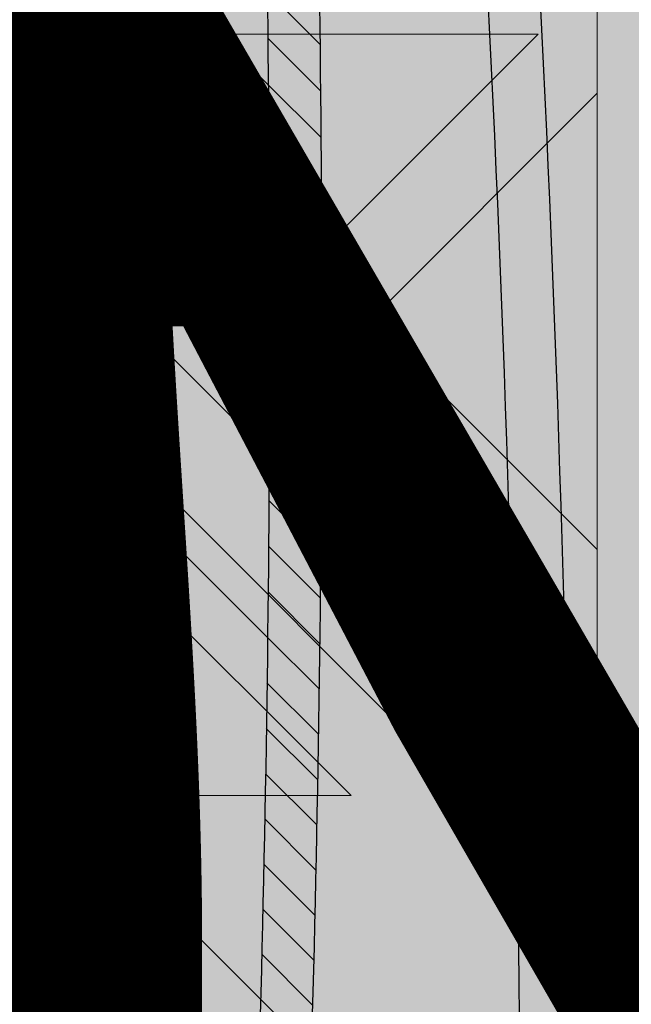
# Model space of a CAD drawing. Units: inches. Extents: x 844 to 2234, y 346 to 1084.
# Tile 82 of 93: x 2006.557 to 2008.425, y 701.365 to 704.373. Entities that reach past the tile are written whole.
import ezdxf

# ---------------------------------------------------------------- set-up
doc = ezdxf.new("R2010")
doc.units = ezdxf.units.IN
doc.header["$MEASUREMENT"] = 0
for name, color, linetype, lineweight in [('A-ANNO-DIMS', 2, 'Continuous', 18), ('furniture', 8, 'Continuous', 18), ('RA-AP-01$0$INT', 35, 'Continuous', 5)]:
    doc.layers.add(name, color=color, linetype=linetype, lineweight=lineweight)
doc.layers.add('RA-AP-01$0$FURN', color=3, linetype='Continuous')
doc.layers.add('RA-AP-01$0$WOOD', color=64, linetype='Continuous')
doc.styles.get("Standard").update_dxf_attribs({"font": 'arial.ttf'})
doc.dimstyles.get("Standard").update_dxf_attribs({"dimtxt": 6, "dimasz": 3, "dimexe": 0.18, "dimexo": 0.0625, "dimgap": 0.09, "dimtad": 0, "dimtih": 1, "dimtoh": 1, "dimdec": 1, "dimzin": 0, "dimdsep": 46, "dimlunit": 3, "dimtxsty": 'Standard', "dimblk": 'ARCHTICK', "dimcen": 0.09, "dimadec": 0, "dimazin": 0, "dimtfac": 1, "dimtdec": 1, "dimtofl": 0, "dimtmove": 0, "dimatfit": 3, "dimfxl": 1, "dimtolj": 1, "dimtzin": 0, "dimarcsym": 0})

# ---------------------------------------------------------------- blocks, each defined once
blk = doc.blocks.new('A$C18D01794')
at = {"layer": 'RA-AP-01$0$INT'}
for points in [[(4.50521, -6.30671), (5.30521, -6.30671), (5.30521, -7.10671), (5.25521, -7.10671), (5.25521, -6.35671), (4.55521, -6.35671), (4.55521, -7.10671), (4.50521, -7.10671)], [(4.50521, -7.90671), (5.30521, -7.90671), (5.30521, -7.10671), (5.25521, -7.10671), (5.25521, -7.85671), (4.55521, -7.85671), (4.55521, -7.10671), (4.50521, -7.10671)]]:
    blk.add_hatch(color=256, dxfattribs=at).paths.add_polyline_path(points)
h = blk.add_hatch(color=256, dxfattribs=at)
h.paths.add_polyline_path([(4.58592, -6.35671), (4.6142, -6.35671), (4.66885, -6.41136), (4.72349, -6.35671), (4.77177, -6.35671), (4.82642, -6.41136), (4.86278, -6.375), (4.8445, -6.35671), (4.86278, -6.35671), (4.90521, -6.39914), (4.94763, -6.35671), (4.96592, -6.35671), (4.94763, -6.375), (4.98399, -6.41136), (5.03864, -6.35671), (5.08692, -6.35671), (5.14157, -6.41136), (5.19621, -6.35671), (5.2245, -6.35671), (4.90521, -6.676)])
h.paths.add_polyline_path([(4.89521, -6.63772), (4.89521, -6.52843), (4.84056, -6.58307)], flags=16)
h.paths.add_polyline_path([(4.91521, -6.63772), (4.96985, -6.58307), (4.91521, -6.52843)], flags=16)
h.paths.add_polyline_path([(4.82642, -6.56893), (4.88106, -6.51429), (4.77177, -6.51429)], flags=16)
h.paths.add_polyline_path([(4.98399, -6.56893), (5.03864, -6.51429), (4.92935, -6.51429)], flags=16)
h.paths.add_polyline_path([(4.88106, -6.49429), (4.82642, -6.43964), (4.77177, -6.49429)], flags=16)
h.paths.add_polyline_path([(4.92935, -6.49429), (5.03864, -6.49429), (4.98399, -6.43964)], flags=16)
h.paths.add_polyline_path([(4.89521, -6.48014), (4.89521, -6.40742), (4.87692, -6.38914), (4.84056, -6.4255)], flags=16)
h.paths.add_polyline_path([(4.91521, -6.48014), (4.96985, -6.4255), (4.93349, -6.38914), (4.91521, -6.40742)], flags=16)
h.paths.add_polyline_path([(4.75763, -6.48014), (4.81228, -6.4255), (4.75763, -6.37085)], flags=16)
h.paths.add_polyline_path([(4.73763, -6.48014), (4.73763, -6.37085), (4.68299, -6.4255)], flags=16)
h.paths.add_polyline_path([(5.05278, -6.48014), (5.05278, -6.37085), (4.99814, -6.4255)], flags=16)
h.paths.add_polyline_path([(5.07278, -6.48014), (5.12742, -6.4255), (5.07278, -6.37085)], flags=16)
h.paths.add_polyline_path([(4.93592, -6.70671), (5.25521, -6.38742), (5.25521, -6.41571), (5.20056, -6.47035), (5.25521, -6.525), (5.25521, -6.57328), (5.20056, -6.62793), (5.23692, -6.66429), (5.25521, -6.646), (5.25521, -6.66429), (5.21278, -6.70671), (5.25521, -6.74914), (5.25521, -6.76742), (5.23692, -6.74914), (5.20056, -6.7855), (5.25521, -6.84014), (5.25521, -6.88843), (5.20056, -6.94307), (5.25521, -6.99772), (5.25521, -7.026)])
h.paths.add_polyline_path([(5.04299, -6.7855), (5.09763, -6.84014), (5.09763, -6.73085)], flags=16)
h.paths.add_polyline_path([(5.02885, -6.77136), (5.08349, -6.71671), (4.9742, -6.71671)], flags=16)
h.paths.add_polyline_path([(5.11763, -6.84014), (5.17228, -6.7855), (5.11763, -6.73085)], flags=16)
h.paths.add_polyline_path([(5.08349, -6.69671), (5.02885, -6.64207), (4.9742, -6.69671)], flags=16)
h.paths.add_polyline_path([(5.13177, -6.85429), (5.18642, -6.79964), (5.24106, -6.85429)], flags=17)
h.paths.add_polyline_path([(5.13177, -6.71671), (5.18642, -6.77136), (5.22278, -6.735), (5.2045, -6.71671)], flags=16)
h.paths.add_polyline_path([(5.09763, -6.68257), (5.09763, -6.57328), (5.04299, -6.62793)], flags=16)
h.paths.add_polyline_path([(5.13177, -6.87429), (5.24106, -6.87429), (5.18642, -6.92893)], flags=17)
h.paths.add_polyline_path([(5.13177, -6.69671), (5.2045, -6.69671), (5.22278, -6.67843), (5.18642, -6.64207)], flags=16)
h.paths.add_polyline_path([(5.11763, -6.68257), (5.17228, -6.62793), (5.11763, -6.57328)], flags=16)
h.paths.add_polyline_path([(5.18642, -6.61378), (5.24106, -6.55914), (5.13177, -6.55914)], flags=16)
h.paths.add_polyline_path([(5.13177, -6.53914), (5.24106, -6.53914), (5.18642, -6.48449)], flags=16)
h.paths.add_polyline_path([(5.25521, -7.08742), (5.25521, -7.10671), (4.55521, -7.10671), (4.55521, -7.08742), (4.90521, -6.73742)])
h.paths.add_polyline_path([(4.98399, -6.84449), (4.92935, -6.89914), (5.03864, -6.89914)], flags=16)
h.paths.add_polyline_path([(4.96985, -6.83035), (4.91521, -6.77571), (4.91521, -6.885)], flags=16)
h.paths.add_polyline_path([(4.92935, -6.91914), (4.98399, -6.97378), (5.03864, -6.91914)], flags=16)
h.paths.add_polyline_path([(5.05278, -6.93328), (4.99814, -6.98793), (5.05278, -7.04257)], flags=16)
h.paths.add_polyline_path([(5.07278, -6.93328), (5.07278, -7.04257), (5.12742, -6.98793)], flags=16)
h.paths.add_polyline_path([(4.89521, -6.77571), (4.84056, -6.83035), (4.89521, -6.885)], flags=16)
h.paths.add_polyline_path([(4.91521, -6.93328), (4.91521, -7.006), (4.93349, -7.02429), (4.96985, -6.98793)], flags=16)
h.paths.add_polyline_path([(4.88106, -6.89914), (4.82642, -6.84449), (4.77177, -6.89914)], flags=16)
h.paths.add_polyline_path([(4.89521, -6.93328), (4.84056, -6.98793), (4.87692, -7.02429), (4.89521, -7.006)], flags=16)
h.paths.add_polyline_path([(4.98399, -7.00207), (4.94763, -7.03843), (4.96592, -7.05671), (5.03864, -7.05671)], flags=16)
h.paths.add_polyline_path([(4.88106, -6.91914), (4.77177, -6.91914), (4.82642, -6.97378)], flags=16)
h.paths.add_polyline_path([(4.90521, -7.01429), (4.86278, -7.05671), (4.94763, -7.05671)], flags=16)
h.paths.add_polyline_path([(5.14157, -7.00207), (5.08692, -7.05671), (5.19621, -7.05671)], flags=16)
h.paths.add_polyline_path([(4.82642, -7.00207), (4.77177, -7.05671), (4.8445, -7.05671), (4.86278, -7.03843)], flags=16)
h.paths.add_polyline_path([(4.81228, -6.98793), (4.75763, -6.93328), (4.75763, -7.04257)], flags=16)
h.paths.add_polyline_path([(4.73763, -6.93328), (4.68299, -6.98793), (4.73763, -7.04257)], flags=16)
h.paths.add_polyline_path([(4.72349, -7.05671), (4.66885, -7.00207), (4.6142, -7.05671)], flags=16)
h.paths.add_polyline_path([(4.59763, -6.70671), (4.55521, -6.66429), (4.55521, -6.646), (4.57349, -6.66429), (4.60985, -6.62793), (4.55521, -6.57328), (4.55521, -6.525), (4.60985, -6.47035), (4.55521, -6.41571), (4.55521, -6.38742), (4.8745, -6.70671), (4.55521, -7.026), (4.55521, -6.99772), (4.60985, -6.94307), (4.55521, -6.88843), (4.55521, -6.84014), (4.60985, -6.7855), (4.57349, -6.74914), (4.55521, -6.76742), (4.55521, -6.74914)])
h.paths.add_polyline_path([(4.71278, -6.73085), (4.71278, -6.84014), (4.76742, -6.7855)], flags=16)
h.paths.add_polyline_path([(4.72692, -6.71671), (4.78157, -6.77136), (4.83621, -6.71671)], flags=16)
h.paths.add_polyline_path([(4.69278, -6.73085), (4.63814, -6.7855), (4.69278, -6.84014)], flags=16)
h.paths.add_polyline_path([(4.72692, -6.69671), (4.83621, -6.69671), (4.78157, -6.64207)], flags=16)
h.paths.add_polyline_path([(4.67864, -6.71671), (4.60592, -6.71671), (4.58763, -6.735), (4.62399, -6.77136)], flags=16)
h.paths.add_polyline_path([(4.71278, -6.68257), (4.76742, -6.62793), (4.71278, -6.57328)], flags=16)
h.paths.add_polyline_path([(4.67864, -6.69671), (4.62399, -6.64207), (4.58763, -6.67843), (4.60592, -6.69671)], flags=16)
h.paths.add_polyline_path([(4.69278, -6.68257), (4.69278, -6.57328), (4.63814, -6.62793)], flags=16)
h.paths.add_polyline_path([(4.62399, -6.79964), (4.67864, -6.85429), (4.56935, -6.85429)], flags=17)
h.paths.add_polyline_path([(4.62399, -6.61378), (4.67864, -6.55914), (4.56935, -6.55914)], flags=16)
h.paths.add_polyline_path([(4.67864, -6.87429), (4.62399, -6.92893), (4.56935, -6.87429)], flags=17)
h.paths.add_polyline_path([(4.67864, -6.53914), (4.62399, -6.48449), (4.56935, -6.53914)], flags=16)
h = blk.add_hatch(color=256, dxfattribs=at)
h.paths.add_polyline_path([(4.58592, -7.85671), (4.6142, -7.85671), (4.66885, -7.80207), (4.72349, -7.85671), (4.77177, -7.85671), (4.82642, -7.80207), (4.86278, -7.83843), (4.8445, -7.85671), (4.86278, -7.85671), (4.90521, -7.81429), (4.94763, -7.85671), (4.96592, -7.85671), (4.94763, -7.83843), (4.98399, -7.80207), (5.03864, -7.85671), (5.08692, -7.85671), (5.14157, -7.80207), (5.19621, -7.85671), (5.2245, -7.85671), (4.90521, -7.53742)])
h.paths.add_polyline_path([(4.89521, -7.57571), (4.89521, -7.685), (4.84056, -7.63035)], flags=16)
h.paths.add_polyline_path([(4.91521, -7.57571), (4.96985, -7.63035), (4.91521, -7.685)], flags=16)
h.paths.add_polyline_path([(4.82642, -7.64449), (4.88106, -7.69914), (4.77177, -7.69914)], flags=16)
h.paths.add_polyline_path([(4.98399, -7.64449), (5.03864, -7.69914), (4.92935, -7.69914)], flags=16)
h.paths.add_polyline_path([(4.88106, -7.71914), (4.82642, -7.77378), (4.77177, -7.71914)], flags=16)
h.paths.add_polyline_path([(4.92935, -7.71914), (5.03864, -7.71914), (4.98399, -7.77378)], flags=16)
h.paths.add_polyline_path([(4.89521, -7.73328), (4.89521, -7.806), (4.87692, -7.82429), (4.84056, -7.78793)], flags=16)
h.paths.add_polyline_path([(4.91521, -7.73328), (4.96985, -7.78793), (4.93349, -7.82429), (4.91521, -7.806)], flags=16)
h.paths.add_polyline_path([(4.75763, -7.73328), (4.81228, -7.78793), (4.75763, -7.84257)], flags=16)
h.paths.add_polyline_path([(4.73763, -7.73328), (4.73763, -7.84257), (4.68299, -7.78793)], flags=16)
h.paths.add_polyline_path([(5.05278, -7.73328), (5.05278, -7.84257), (4.99814, -7.78793)], flags=16)
h.paths.add_polyline_path([(5.07278, -7.73328), (5.12742, -7.78793), (5.07278, -7.84257)], flags=16)
h.paths.add_polyline_path([(4.93592, -7.50671), (5.25521, -7.826), (5.25521, -7.79772), (5.20056, -7.74307), (5.25521, -7.68843), (5.25521, -7.64014), (5.20056, -7.5855), (5.23692, -7.54914), (5.25521, -7.56742), (5.25521, -7.54914), (5.21278, -7.50671), (5.25521, -7.46429), (5.25521, -7.446), (5.23692, -7.46429), (5.20056, -7.42793), (5.25521, -7.37328), (5.25521, -7.325), (5.20056, -7.27035), (5.25521, -7.21571), (5.25521, -7.18742)])
h.paths.add_polyline_path([(5.04299, -7.42793), (5.09763, -7.37328), (5.09763, -7.48257)], flags=16)
h.paths.add_polyline_path([(5.02885, -7.44207), (5.08349, -7.49671), (4.9742, -7.49671)], flags=16)
h.paths.add_polyline_path([(5.11763, -7.37328), (5.17228, -7.42793), (5.11763, -7.48257)], flags=16)
h.paths.add_polyline_path([(5.08349, -7.51671), (5.02885, -7.57136), (4.9742, -7.51671)], flags=16)
h.paths.add_polyline_path([(5.13177, -7.35914), (5.18642, -7.41378), (5.24106, -7.35914)], flags=17)
h.paths.add_polyline_path([(5.13177, -7.49671), (5.18642, -7.44207), (5.22278, -7.47843), (5.2045, -7.49671)], flags=16)
h.paths.add_polyline_path([(5.09763, -7.53085), (5.09763, -7.64014), (5.04299, -7.5855)], flags=16)
h.paths.add_polyline_path([(5.13177, -7.33914), (5.24106, -7.33914), (5.18642, -7.28449)], flags=17)
h.paths.add_polyline_path([(5.13177, -7.51671), (5.2045, -7.51671), (5.22278, -7.535), (5.18642, -7.57136)], flags=16)
h.paths.add_polyline_path([(5.11763, -7.53085), (5.17228, -7.5855), (5.11763, -7.64014)], flags=16)
h.paths.add_polyline_path([(5.18642, -7.59964), (5.24106, -7.65429), (5.13177, -7.65429)], flags=16)
h.paths.add_polyline_path([(5.13177, -7.67429), (5.24106, -7.67429), (5.18642, -7.72893)], flags=16)
h.paths.add_polyline_path([(5.25521, -7.126), (5.25521, -7.10671), (4.55521, -7.10671), (4.55521, -7.126), (4.90521, -7.476)])
h.paths.add_polyline_path([(4.98399, -7.36893), (4.92935, -7.31429), (5.03864, -7.31429)], flags=16)
h.paths.add_polyline_path([(4.96985, -7.38307), (4.91521, -7.43772), (4.91521, -7.32843)], flags=16)
h.paths.add_polyline_path([(4.92935, -7.29429), (4.98399, -7.23964), (5.03864, -7.29429)], flags=16)
h.paths.add_polyline_path([(5.05278, -7.28014), (4.99814, -7.2255), (5.05278, -7.17085)], flags=16)
h.paths.add_polyline_path([(5.07278, -7.28014), (5.07278, -7.17085), (5.12742, -7.2255)], flags=16)
h.paths.add_polyline_path([(4.89521, -7.43772), (4.84056, -7.38307), (4.89521, -7.32843)], flags=16)
h.paths.add_polyline_path([(4.91521, -7.28014), (4.91521, -7.20742), (4.93349, -7.18914), (4.96985, -7.2255)], flags=16)
h.paths.add_polyline_path([(4.88106, -7.31429), (4.82642, -7.36893), (4.77177, -7.31429)], flags=16)
h.paths.add_polyline_path([(4.89521, -7.28014), (4.84056, -7.2255), (4.87692, -7.18914), (4.89521, -7.20742)], flags=16)
h.paths.add_polyline_path([(4.98399, -7.21136), (4.94763, -7.175), (4.96592, -7.15671), (5.03864, -7.15671)], flags=16)
h.paths.add_polyline_path([(4.88106, -7.29429), (4.77177, -7.29429), (4.82642, -7.23964)], flags=16)
h.paths.add_polyline_path([(4.90521, -7.19914), (4.86278, -7.15671), (4.94763, -7.15671)], flags=16)
h.paths.add_polyline_path([(5.14157, -7.21136), (5.08692, -7.15671), (5.19621, -7.15671)], flags=16)
h.paths.add_polyline_path([(4.82642, -7.21136), (4.77177, -7.15671), (4.8445, -7.15671), (4.86278, -7.175)], flags=16)
h.paths.add_polyline_path([(4.81228, -7.2255), (4.75763, -7.28014), (4.75763, -7.17085)], flags=16)
h.paths.add_polyline_path([(4.73763, -7.28014), (4.68299, -7.2255), (4.73763, -7.17085)], flags=16)
h.paths.add_polyline_path([(4.72349, -7.15671), (4.66885, -7.21136), (4.6142, -7.15671)], flags=16)
h.paths.add_polyline_path([(4.59763, -7.50671), (4.55521, -7.54914), (4.55521, -7.56742), (4.57349, -7.54914), (4.60985, -7.5855), (4.55521, -7.64014), (4.55521, -7.68843), (4.60985, -7.74307), (4.55521, -7.79772), (4.55521, -7.826), (4.8745, -7.50671), (4.55521, -7.18742), (4.55521, -7.21571), (4.60985, -7.27035), (4.55521, -7.325), (4.55521, -7.37328), (4.60985, -7.42793), (4.57349, -7.46429), (4.55521, -7.446), (4.55521, -7.46429)])
h.paths.add_polyline_path([(4.71278, -7.48257), (4.71278, -7.37328), (4.76742, -7.42793)], flags=16)
h.paths.add_polyline_path([(4.72692, -7.49671), (4.78157, -7.44207), (4.83621, -7.49671)], flags=16)
h.paths.add_polyline_path([(4.69278, -7.48257), (4.63814, -7.42793), (4.69278, -7.37328)], flags=16)
h.paths.add_polyline_path([(4.72692, -7.51671), (4.83621, -7.51671), (4.78157, -7.57136)], flags=16)
h.paths.add_polyline_path([(4.67864, -7.49671), (4.60592, -7.49671), (4.58763, -7.47843), (4.62399, -7.44207)], flags=16)
h.paths.add_polyline_path([(4.71278, -7.53085), (4.76742, -7.5855), (4.71278, -7.64014)], flags=16)
h.paths.add_polyline_path([(4.67864, -7.51671), (4.62399, -7.57136), (4.58763, -7.535), (4.60592, -7.51671)], flags=16)
h.paths.add_polyline_path([(4.69278, -7.53085), (4.69278, -7.64014), (4.63814, -7.5855)], flags=16)
h.paths.add_polyline_path([(4.62399, -7.41378), (4.67864, -7.35914), (4.56935, -7.35914)], flags=17)
h.paths.add_polyline_path([(4.62399, -7.59964), (4.67864, -7.65429), (4.56935, -7.65429)], flags=16)
h.paths.add_polyline_path([(4.67864, -7.33914), (4.62399, -7.28449), (4.56935, -7.33914)], flags=17)
h.paths.add_polyline_path([(4.67864, -7.67429), (4.62399, -7.72893), (4.56935, -7.67429)], flags=16)
h = blk.add_hatch(color=256, dxfattribs=at)
h.paths.add_polyline_path([(4.90521, -7.53742), (4.8745, -7.50671), (4.55521, -7.826), (4.55521, -7.85671), (4.58592, -7.85671)])
h.paths.add_polyline_path([(4.93592, -7.50671), (4.90521, -7.53742), (5.2245, -7.85671), (5.25521, -7.85671), (5.25521, -7.826)])
h.paths.add_polyline_path([(5.25521, -7.18742), (5.25521, -7.126), (4.90521, -7.476), (4.93592, -7.50671)])
h.paths.add_polyline_path([(4.8745, -7.50671), (4.90521, -7.476), (4.55521, -7.126), (4.55521, -7.18742)])
h = blk.add_hatch(color=256, dxfattribs=at)
h.paths.add_polyline_path([(4.89521, -7.32843), (4.84056, -7.38307), (4.89521, -7.43772)])
h.paths.add_polyline_path([(4.91521, -7.43772), (4.96985, -7.38307), (4.91521, -7.32843)])
h.paths.add_polyline_path([(4.92935, -7.31429), (4.98399, -7.36893), (5.03864, -7.31429)])
h.paths.add_polyline_path([(5.03864, -7.29429), (4.98399, -7.23964), (4.92935, -7.29429)])
h.paths.add_polyline_path([(4.96985, -7.2255), (4.93349, -7.18914), (4.91521, -7.20742), (4.91521, -7.28014)])
h.paths.add_polyline_path([(4.96592, -7.15671), (4.94763, -7.175), (4.98399, -7.21136), (5.03864, -7.15671)])
h.paths.add_polyline_path([(4.99814, -7.2255), (5.05278, -7.28014), (5.05278, -7.17085)])
h.paths.add_polyline_path([(5.07278, -7.28014), (5.12742, -7.2255), (5.07278, -7.17085)])
h.paths.add_polyline_path([(5.19621, -7.15671), (5.08692, -7.15671), (5.14157, -7.21136)])
h.paths.add_polyline_path([(4.86278, -7.15671), (4.90521, -7.19914), (4.94763, -7.15671)])
h.paths.add_polyline_path([(4.89521, -7.28014), (4.89521, -7.20742), (4.87692, -7.18914), (4.84056, -7.2255)])
h.paths.add_polyline_path([(4.82642, -7.23964), (4.77177, -7.29429), (4.88106, -7.29429)])
h.paths.add_polyline_path([(4.77177, -7.31429), (4.82642, -7.36893), (4.88106, -7.31429)])
h.paths.add_polyline_path([(4.75763, -7.28014), (4.81228, -7.2255), (4.75763, -7.17085)])
h.paths.add_polyline_path([(4.86278, -7.175), (4.8445, -7.15671), (4.77177, -7.15671), (4.82642, -7.21136)])
h.paths.add_polyline_path([(4.68299, -7.2255), (4.73763, -7.28014), (4.73763, -7.17085)])
h.paths.add_polyline_path([(4.72349, -7.15671), (4.6142, -7.15671), (4.66885, -7.21136)])
h = blk.add_hatch(color=256, dxfattribs=at)
h.paths.add_polyline_path([(4.78157, -7.44207), (4.83621, -7.49671), (4.72692, -7.49671)])
h.paths.add_polyline_path([(4.83621, -7.51671), (4.78157, -7.57136), (4.72692, -7.51671)])
h.paths.add_polyline_path([(4.76742, -7.5855), (4.71278, -7.64014), (4.71278, -7.53085)])
h.paths.add_polyline_path([(4.69278, -7.53085), (4.69278, -7.64014), (4.63814, -7.5855)])
h.paths.add_polyline_path([(4.67864, -7.51671), (4.62399, -7.57136), (4.58763, -7.535), (4.60592, -7.51671)])
h.paths.add_polyline_path([(4.57349, -7.54914), (4.60985, -7.5855), (4.55521, -7.64014), (4.55521, -7.56742)])
h.paths.add_polyline_path([(4.62399, -7.59964), (4.67864, -7.65429), (4.56935, -7.65429)])
h.paths.add_polyline_path([(4.67864, -7.67429), (4.62399, -7.72893), (4.56935, -7.67429)])
h.paths.add_polyline_path([(4.60985, -7.74307), (4.55521, -7.79772), (4.55521, -7.68843)])
h.paths.add_polyline_path([(4.59763, -7.50671), (4.55521, -7.54914), (4.55521, -7.46429)])
h.paths.add_polyline_path([(4.67864, -7.49671), (4.60592, -7.49671), (4.58763, -7.47843), (4.62399, -7.44207)])
h.paths.add_polyline_path([(4.69278, -7.37328), (4.69278, -7.48257), (4.63814, -7.42793)])
h.paths.add_polyline_path([(4.76742, -7.42793), (4.71278, -7.48257), (4.71278, -7.37328)])
h.paths.add_polyline_path([(4.67864, -7.35914), (4.62399, -7.41378), (4.56935, -7.35914)])
h.paths.add_polyline_path([(4.60985, -7.42793), (4.57349, -7.46429), (4.55521, -7.446), (4.55521, -7.37328)])
h.paths.add_polyline_path([(4.62399, -7.28449), (4.67864, -7.33914), (4.56935, -7.33914)])
h.paths.add_polyline_path([(4.60985, -7.27035), (4.55521, -7.325), (4.55521, -7.21571)])
for p, q in [((4.55521, -7.10671), (4.55521, -6.35671)), ((4.55521, -7.10671), (4.55521, -7.85671)), ((4.90521, -7.476), (4.55521, -7.126)), ((4.72349, -7.15671), (4.6142, -7.15671)), ((4.6142, -7.15671), (4.66885, -7.21136)), ((4.72349, -7.15671), (4.66885, -7.21136)), ((4.73763, -7.17085), (4.68299, -7.2255)), ((4.8745, -7.50671), (4.55521, -7.18742)), ((4.55521, -7.21571), (4.60985, -7.27035)), ((4.55521, -7.325), (4.55521, -7.21571)), ((4.68299, -7.2255), (4.73763, -7.28014)), ((4.55521, -7.325), (4.60985, -7.27035)), ((4.56935, -7.33914), (4.62399, -7.28449)), ((4.62399, -7.28449), (4.67864, -7.33914)), ((4.67864, -7.33914), (4.56935, -7.33914))]:
    blk.add_line(p, q, dxfattribs=at)
blk = doc.blocks.new('A$C32926AE1')
at = {"layer": 'RA-AP-01$0$WOOD'}
h = blk.add_hatch(color=256, dxfattribs=at)
h.dxf.hatch_style = 1
h.paths.add_polyline_path([(5.15743, 4.57348, -0.100949), (5.1554, 4.59337, -0.184266), (5.17225, 4.6388, 0.205661), (5.17956, 4.66132, 0.361434), (5.13435, 4.70652, 0.205661), (5.11183, 4.69921, -0.184266), (5.0664, 4.68237, -0.105531), (5.04566, 4.68467, 0.156764), (4.76389, 4.68467, -0.105531), (4.74314, 4.68237, -0.184266), (4.69771, 4.69921, 0.205661), (4.67519, 4.70652, 0.361434), (4.62998, 4.66132, 0.205661), (4.63729, 4.6388, -0.184266), (4.65414, 4.59337, -0.100949), (4.65211, 4.57348, 0.02141), (4.62975, 4.15671, 0.02141), (4.65211, 3.73994, -0.100949), (4.65414, 3.72006, -0.184266), (4.63729, 3.67463, 0.205661), (4.62998, 3.65211, 0.361434), (4.67519, 3.6069, 0.205661), (4.69771, 3.61421, -0.184266), (4.74314, 3.63106, -0.105531), (4.76389, 3.62875, 0.156764), (5.04566, 3.62875, -0.105531), (5.0664, 3.63106, -0.184266), (5.11183, 3.61421, 0.205661), (5.13435, 3.6069, 0.361434), (5.17956, 3.65211, 0.205661), (5.17225, 3.67463, -0.184266), (5.1554, 3.72006, -0.100949), (5.15743, 3.73994, 0.02141), (5.17979, 4.15671, 0.02141)])
h.paths.add_polyline_path([(4.63975, 4.15671, 0.021354), (4.66197, 3.74189, -0.094076), (4.66414, 3.71961, -0.182482), (4.64481, 3.66804, 0.205661), (4.63994, 3.65302, 0.361434), (4.67611, 3.61686, 0.205661), (4.69112, 3.62173, -0.182482), (4.7427, 3.64106, -0.102989), (4.76699, 3.63826, 0.156709), (5.04255, 3.63826, -0.102989), (5.06685, 3.64106, -0.182482), (5.11842, 3.62173, 0.205661), (5.13344, 3.61686, 0.361434), (5.1696, 3.65302, 0.205661), (5.16473, 3.66804, -0.182482), (5.1454, 3.71961, -0.094076), (5.14757, 3.74189, 0.021354), (5.16979, 4.15671, 0.021354), (5.14757, 4.57154, -0.094076), (5.1454, 4.59381, -0.182482), (5.16473, 4.64539, 0.205661), (5.1696, 4.6604, 0.361434), (5.13344, 4.69657, 0.205661), (5.11842, 4.69169, -0.182482), (5.06685, 4.67236, -0.102989), (5.04255, 4.67517, 0.156709), (4.76699, 4.67517, -0.102989), (4.7427, 4.67236, -0.182482), (4.69112, 4.69169, 0.205661), (4.67611, 4.69657, 0.361434), (4.63994, 4.6604, 0.205661), (4.64481, 4.64539, -0.182482), (4.66414, 4.59381, -0.094076), (4.66197, 4.57154, 0.021354)], flags=16)
h.paths.add_polyline_path([(5.12979, 4.43217, -0.014166), (5.13015, 4.15693, -0.014166), (5.12979, 3.88169, -0.078525), (5.1098, 3.75514, 0.094597), (5.10541, 3.7179, 0.104317), (5.11607, 3.67039, 0.104317), (5.06856, 3.68105, 0.094597), (5.03132, 3.67666, -0.158024), (4.77823, 3.67666, 0.094597), (4.74098, 3.68105, 0.104317), (4.69347, 3.67039, 0.104317), (4.70413, 3.7179, 0.094597), (4.69975, 3.75514, -0.078525), (4.67975, 3.88169, -0.014166), (4.67939, 4.15693, -0.014166), (4.67975, 4.43217, -0.078525), (4.69975, 4.55871, 0.094597), (4.70413, 4.59596, 0.104317), (4.69347, 4.64347, 0.104317), (4.74098, 4.6328, 0.094597), (4.77823, 4.63719, -0.158024), (5.03132, 4.63719, 0.094597), (5.06856, 4.6328, 0.104317), (5.11607, 4.64347, 0.104317), (5.10541, 4.59596, 0.094597), (5.1098, 4.55871, -0.078525)], flags=0)
h.paths.add_polyline_path([(5.11979, 4.43226, -0.0142), (5.12016, 4.15693, -0.0142), (5.11979, 3.8816, -0.078489), (5.10027, 3.75819, 0.094014), (5.09541, 3.71748, 0.060627), (5.09962, 3.68684, 0.060627), (5.06898, 3.69105, 0.094014), (5.02827, 3.68619, -0.158071), (4.78127, 3.68619, 0.094014), (4.74056, 3.69105, 0.060627), (4.70993, 3.68684, 0.060627), (4.71413, 3.71748, 0.094014), (4.70927, 3.75819, -0.078489), (4.68975, 3.8816, -0.0142), (4.68939, 4.15693, -0.0142), (4.68975, 4.43226, -0.078489), (4.70927, 4.55566, 0.094014), (4.71413, 4.59638, 0.060627), (4.70993, 4.62701, 0.060627), (4.74056, 4.62281, 0.094014), (4.78127, 4.62767, -0.158071), (5.02827, 4.62767, 0.094014), (5.06898, 4.62281, 0.060627), (5.09962, 4.62701, 0.060627), (5.09541, 4.59638, 0.094014), (5.10027, 4.55566, -0.078489)], flags=0)
h.paths.add_polyline_path([(5.06979, 4.43022, -0.014242), (5.07017, 4.15693, -0.014242), (5.06979, 3.88364, -0.080061), (5.05266, 3.77346, 0.052642), (5.04591, 3.74055, 0.052642), (5.013, 3.7338, -0.158303), (4.79655, 3.7338, 0.052642), (4.76363, 3.74055, 0.052642), (4.75688, 3.77346, -0.080061), (4.73975, 3.88364, -0.014242), (4.73937, 4.15693, -0.014242), (4.73975, 4.43022, -0.080061), (4.75688, 4.54039, 0.052642), (4.76363, 4.5733, 0.052642), (4.79655, 4.58006, -0.158303), (5.013, 4.58006, 0.052642), (5.04591, 4.5733, 0.052642), (5.05266, 4.54039, -0.080061)], flags=0)
h.paths.add_polyline_path([(5.04979, 4.43038, -0.01431), (5.05018, 4.15693, -0.01431), (5.04979, 3.88347, -0.080069), (5.03362, 3.77958, 0.030626), (5.02824, 3.75822, 0.030626), (5.00688, 3.75284, -0.158398), (4.80266, 3.75284, 0.030626), (4.7813, 3.75822, 0.030626), (4.77592, 3.77958, -0.080069), (4.75975, 3.88347, -0.01431), (4.75936, 4.15693, -0.01431), (4.75975, 4.43038, -0.080069), (4.77592, 4.53427, 0.030626), (4.7813, 4.55564, 0.030626), (4.80266, 4.56102, -0.158398), (5.00688, 4.56102, 0.030626), (5.02824, 4.55564, 0.030626), (5.03362, 4.53427, -0.080069)], flags=0)
h.paths.add_polyline_path([(4.99977, 4.42817, -0.014344), (5.0002, 4.15693, -0.014344), (4.99977, 3.88568, -0.078464), (4.98736, 3.7991, -0.150605), (4.82219, 3.7991, -0.078464), (4.80978, 3.88568, -0.014344), (4.80934, 4.15693, -0.014344), (4.80978, 4.42817, -0.078464), (4.82219, 4.51475, -0.150605), (4.98736, 4.51475, -0.078464)], flags=0)
h.paths.add_polyline_path([(4.97976, 4.42764, -0.014377), (4.98021, 4.15693, -0.014377), (4.97976, 3.88621, -0.068924), (4.97118, 3.81528, -0.129665), (4.83836, 3.81528, -0.068924), (4.82979, 3.88621, -0.014377), (4.82934, 4.15693, -0.014377), (4.82979, 4.42764, -0.068924), (4.83836, 4.49858, -0.129665), (4.97118, 4.49858, -0.068924)], flags=0)
h = blk.add_hatch(color=256, dxfattribs=at)
h.dxf.hatch_style = 1
h.paths.add_polyline_path([(5.1454, 4.59381, -0.182482), (5.16473, 4.64539, 0.205661), (5.1696, 4.6604, 0.361434), (5.13344, 4.69657, 0.205661), (5.11842, 4.69169, -0.182482), (5.06685, 4.67236, -0.102989), (5.04255, 4.67517, 0.156709), (4.76699, 4.67517, -0.102989), (4.7427, 4.67236, -0.182482), (4.69112, 4.69169, 0.205661), (4.67611, 4.69657, 0.361434), (4.63994, 4.6604, 0.205661), (4.64481, 4.64539, -0.182482), (4.66414, 4.59381, -0.094076), (4.66197, 4.57154, 0.021354), (4.63975, 4.15671, 0.021354), (4.66197, 3.74189, -0.094076), (4.66414, 3.71961, -0.182482), (4.64481, 3.66804, 0.205661), (4.63994, 3.65302, 0.361434), (4.67611, 3.61686, 0.205661), (4.69112, 3.62173, -0.182482), (4.7427, 3.64106, -0.102989), (4.76699, 3.63826, 0.156709), (5.04255, 3.63826, -0.102989), (5.06685, 3.64106, -0.182482), (5.11842, 3.62173, 0.205661), (5.13344, 3.61686, 0.361434), (5.1696, 3.65302, 0.205661), (5.16473, 3.66804, -0.182482), (5.1454, 3.71961, -0.094076), (5.14757, 3.74189, 0.021354), (5.16979, 4.15671, 0.021354), (5.14757, 4.57154, -0.094076)])
h.paths.add_polyline_path([(5.1098, 4.55871, -0.078525), (5.12979, 4.43217, -0.014166), (5.13015, 4.15693, -0.014166), (5.12979, 3.88169, -0.078525), (5.1098, 3.75514, 0.094597), (5.10541, 3.7179, 0.104317), (5.11607, 3.67039, 0.104317), (5.06856, 3.68105, 0.094597), (5.03132, 3.67666, -0.158024), (4.77823, 3.67666, 0.094597), (4.74098, 3.68105, 0.104317), (4.69347, 3.67039, 0.104317), (4.70413, 3.7179, 0.094597), (4.69975, 3.75514, -0.078525), (4.67975, 3.88169, -0.014166), (4.67939, 4.15693, -0.014166), (4.67975, 4.43217, -0.078525), (4.69975, 4.55871, 0.094597), (4.70413, 4.59596, 0.104317), (4.69347, 4.64347, 0.104317), (4.74098, 4.6328, 0.094597), (4.77823, 4.63719, -0.158024), (5.03132, 4.63719, 0.094597), (5.06856, 4.6328, 0.104317), (5.11607, 4.64347, 0.104317), (5.10541, 4.59596, 0.094597)], flags=16)
h.paths.add_polyline_path([(5.10027, 4.55566, -0.078489), (5.11979, 4.43226, -0.0142), (5.12016, 4.15693, -0.0142), (5.11979, 3.8816, -0.078489), (5.10027, 3.75819, 0.094014), (5.09541, 3.71748, 0.060627), (5.09962, 3.68684, 0.060627), (5.06898, 3.69105, 0.094014), (5.02827, 3.68619, -0.158071), (4.78127, 3.68619, 0.094014), (4.74056, 3.69105, 0.060627), (4.70993, 3.68684, 0.060627), (4.71413, 3.71748, 0.094014), (4.70927, 3.75819, -0.078489), (4.68975, 3.8816, -0.0142), (4.68939, 4.15693, -0.0142), (4.68975, 4.43226, -0.078489), (4.70927, 4.55566, 0.094014), (4.71413, 4.59638, 0.060627), (4.70993, 4.62701, 0.060627), (4.74056, 4.62281, 0.094014), (4.78127, 4.62767, -0.158071), (5.02827, 4.62767, 0.094014), (5.06898, 4.62281, 0.060627), (5.09962, 4.62701, 0.060627), (5.09541, 4.59638, 0.094014)], flags=0)
h.paths.add_polyline_path([(5.04591, 4.5733, 0.052642), (5.05266, 4.54039, -0.080061), (5.06979, 4.43022, -0.014242), (5.07017, 4.15693, -0.014242), (5.06979, 3.88364, -0.080061), (5.05266, 3.77346, 0.052642), (5.04591, 3.74055, 0.052642), (5.013, 3.7338, -0.158303), (4.79655, 3.7338, 0.052642), (4.76363, 3.74055, 0.052642), (4.75688, 3.77346, -0.080061), (4.73975, 3.88364, -0.014242), (4.73937, 4.15693, -0.014242), (4.73975, 4.43022, -0.080061), (4.75688, 4.54039, 0.052642), (4.76363, 4.5733, 0.052642), (4.79655, 4.58006, -0.158303), (5.013, 4.58006, 0.052642)], flags=0)
h.paths.add_polyline_path([(5.02824, 4.55564, 0.030626), (5.03362, 4.53427, -0.080069), (5.04979, 4.43038, -0.01431), (5.05018, 4.15693, -0.01431), (5.04979, 3.88347, -0.080069), (5.03362, 3.77958, 0.030626), (5.02824, 3.75822, 0.030626), (5.00688, 3.75284, -0.158398), (4.80266, 3.75284, 0.030626), (4.7813, 3.75822, 0.030626), (4.77592, 3.77958, -0.080069), (4.75975, 3.88347, -0.01431), (4.75936, 4.15693, -0.01431), (4.75975, 4.43038, -0.080069), (4.77592, 4.53427, 0.030626), (4.7813, 4.55564, 0.030626), (4.80266, 4.56102, -0.158398), (5.00688, 4.56102, 0.030626)], flags=0)
h.paths.add_polyline_path([(4.98736, 4.51475, -0.078464), (4.99977, 4.42817, -0.014344), (5.0002, 4.15693, -0.014344), (4.99977, 3.88568, -0.078464), (4.98736, 3.7991, -0.150605), (4.82219, 3.7991, -0.078464), (4.80978, 3.88568, -0.014344), (4.80934, 4.15693, -0.014344), (4.80978, 4.42817, -0.078464), (4.82219, 4.51475, -0.150605)], flags=0)
h.paths.add_polyline_path([(4.97118, 4.49858, -0.068924), (4.97976, 4.42764, -0.014377), (4.98021, 4.15693, -0.014377), (4.97976, 3.88621, -0.068924), (4.97118, 3.81528, -0.129665), (4.83836, 3.81528, -0.068924), (4.82979, 3.88621, -0.014377), (4.82934, 4.15693, -0.014377), (4.82979, 4.42764, -0.068924), (4.83836, 4.49858, -0.129665)], flags=0)
h = blk.add_hatch(dxfattribs=at)
h.set_pattern_fill('ANSI31', color=256, scale=0.05, style=0)
h.paths.add_polyline_path([(5.13015, 4.15693, 0.014166), (5.12979, 4.43217, 0.077783), (5.11017, 4.55756, -0.097652), (5.10541, 4.59596, -0.104317), (5.11607, 4.64347), (5.09962, 4.62701, 0.060627), (5.09541, 4.59638, 0.094014), (5.10027, 4.55566, -0.078489), (5.11979, 4.43226, -0.0142), (5.12016, 4.15693, -0.0142), (5.11979, 3.8816, -0.078489), (5.10027, 3.75819, 0.094014), (5.09541, 3.71748, 0.060627), (5.09962, 3.68684), (5.11607, 3.67039, -0.104317), (5.10541, 3.7179, -0.097652), (5.11017, 3.7563, 0.077783), (5.12979, 3.88169, 0.014166)])
h.paths.add_polyline_path([(5.03016, 3.67629, -0.097652), (5.06856, 3.68105, -0.104317), (5.11607, 3.67039), (5.09962, 3.68684, 0.060627), (5.06898, 3.69105, 0.094014), (5.02827, 3.68619, -0.158071), (4.78127, 3.68619, 0.094014), (4.74056, 3.69105, 0.060627), (4.70993, 3.68684), (4.69347, 3.67039, -0.104317), (4.74098, 3.68105, -0.097652), (4.77938, 3.67629, 0.156513)])
h.paths.add_polyline_path([(4.68975, 3.8816, -0.0142), (4.68939, 4.15693, -0.0142), (4.68975, 4.43226, -0.078489), (4.70927, 4.55566, 0.094014), (4.71413, 4.59638, 0.060627), (4.70993, 4.62701), (4.69347, 4.64347, -0.104317), (4.70413, 4.59596, -0.097652), (4.69937, 4.55756, 0.077783), (4.67975, 4.43217, 0.014166), (4.67939, 4.15693, 0.014166), (4.67975, 3.88169, 0.077783), (4.69937, 3.7563, -0.097652), (4.70413, 3.7179, -0.104317), (4.69347, 3.67039), (4.70993, 3.68684, 0.060627), (4.71413, 3.71748, 0.094014), (4.70927, 3.75819, -0.078489)])
h.paths.add_polyline_path([(4.77938, 4.63756, -0.097652), (4.74098, 4.6328, -0.104317), (4.69347, 4.64347), (4.70993, 4.62701, 0.060627), (4.74056, 4.62281, 0.094014), (4.78127, 4.62767, -0.158071), (5.02827, 4.62767, 0.094014), (5.06898, 4.62281, 0.060627), (5.09962, 4.62701), (5.11607, 4.64347, -0.104317), (5.06856, 4.6328, -0.097652), (5.03016, 4.63756, 0.156513)])
h = blk.add_hatch(dxfattribs=at)
h.set_pattern_fill('ANSI32', color=256, scale=0.2, style=0)
h.paths.add_polyline_path([(5.11979, 4.43226, 0.077702), (5.10066, 4.55447, -0.09689), (5.09541, 4.59638, -0.060627), (5.09962, 4.62701, -0.060627), (5.06898, 4.62281, -0.09689), (5.02707, 4.62805, 0.156466), (4.78247, 4.62805, -0.09689), (4.74056, 4.62281, -0.060627), (4.70993, 4.62701, -0.060627), (4.71413, 4.59638, -0.09689), (4.70888, 4.55447, 0.077702), (4.68975, 4.43226, 0.0142), (4.68939, 4.15693, 0.0142), (4.68975, 3.8816, 0.077702), (4.70888, 3.75939, -0.09689), (4.71413, 3.71748, -0.060627), (4.70993, 3.68684, -0.060627), (4.74056, 3.69105, -0.09689), (4.78247, 3.6858, 0.156466), (5.02707, 3.6858, -0.09689), (5.06898, 3.69105, -0.060627), (5.09962, 3.68684, -0.060627), (5.09541, 3.71748, -0.09689), (5.10066, 3.75939, 0.077702), (5.11979, 3.8816, 0.0142), (5.12016, 4.15693, 0.0142)])
h.paths.add_polyline_path([(5.07017, 4.15693, -0.014242), (5.06979, 3.88364, -0.080061), (5.05266, 3.77346, 0.052642), (5.04591, 3.74055, 0.052642), (5.013, 3.7338, -0.158303), (4.79655, 3.7338, 0.052642), (4.76363, 3.74055, 0.052642), (4.75688, 3.77346, -0.080061), (4.73975, 3.88364, -0.014242), (4.73937, 4.15693, -0.014242), (4.73975, 4.43022, -0.080061), (4.75688, 4.54039, 0.052642), (4.76363, 4.5733, 0.052642), (4.79655, 4.58006, -0.158303), (5.013, 4.58006, 0.052642), (5.04591, 4.5733, 0.052642), (5.05266, 4.54039, -0.080061), (5.06979, 4.43022, -0.014242)], flags=16)
h.paths.add_polyline_path([(5.05018, 4.15693, -0.01431), (5.04979, 3.88347, -0.080069), (5.03362, 3.77958, 0.030626), (5.02824, 3.75822, 0.030626), (5.00688, 3.75284, -0.158398), (4.80266, 3.75284, 0.030626), (4.7813, 3.75822, 0.030626), (4.77592, 3.77958, -0.080069), (4.75975, 3.88347, -0.01431), (4.75936, 4.15693, -0.01431), (4.75975, 4.43038, -0.080069), (4.77592, 4.53427, 0.030626), (4.7813, 4.55564, 0.030626), (4.80266, 4.56102, -0.158398), (5.00688, 4.56102, 0.030626), (5.02824, 4.55564, 0.030626), (5.03362, 4.53427, -0.080069), (5.04979, 4.43038, -0.01431)], flags=0)
h.paths.add_polyline_path([(5.0002, 4.15693, -0.014344), (4.99977, 3.88568, -0.078464), (4.98736, 3.7991, -0.150605), (4.82219, 3.7991, -0.078464), (4.80978, 3.88568, -0.014344), (4.80934, 4.15693, -0.014344), (4.80978, 4.42817, -0.078464), (4.82219, 4.51475, -0.150605), (4.98736, 4.51475, -0.078464), (4.99977, 4.42817, -0.014344)], flags=0)
h.paths.add_polyline_path([(4.98021, 4.15693, -0.014377), (4.97976, 3.88621, -0.068924), (4.97118, 3.81528, -0.129665), (4.83836, 3.81528, -0.068924), (4.82979, 3.88621, -0.014377), (4.82934, 4.15693, -0.014377), (4.82979, 4.42764, -0.068924), (4.83836, 4.49858, -0.129665), (4.97118, 4.49858, -0.068924), (4.97976, 4.42764, -0.014377)], flags=0)
for centre, radius, start, end in [((9.50522, 4.10408), 4.87575, 174.47541, 179.3815), ((9.50522, 4.10408), 4.86575, 174.48704, 179.3815), ((9.53595, 4.28823), 4.85833, 178.30224, 181.54738), ((9.53595, 4.28823), 4.84835, 178.3067, 181.55184)]:
    blk.add_arc(centre, radius, start, end, dxfattribs=at)
blk = doc.blocks.new('A$C5D2F253E')
at = {"layer": 'RA-AP-01$0$FURN', "xscale": -0.7999999999883585, "yscale": 0.7999999999883585, "zscale": 0.8, "rotation": 90}
blk.add_blockref('A$C18D01794', (-5.68776, 4.75792), dxfattribs=at)
at = {"layer": 'RA-AP-01$0$WOOD', "rotation": 270}
blk.add_blockref('A$C32926AE1', (-4.16134, 5.73853), dxfattribs=at)
blk = doc.blocks.new('_ArchTick')
at = {"color": 0, "linetype": 'ByBlock', "const_width": 0.15}
blk.add_lwpolyline([(-0.5, -0.5), (0.5, 0.5)], dxfattribs=at)
blk = doc.blocks.new('*D121')
at = {"layer": 'A-ANNO-DIMS', "color": 0, "lineweight": -2, "transparency": 16777216}
for p, q in [((2030.272, 734.2626), (2040.2453, 734.2626)), ((2040.0653, 734.2626), (2040.0653, 704.6044)), ((2040.0653, 668.5574), (2040.0653, 698.2156)), ((2030.272, 668.5574), (2040.2453, 668.5574))]:
    blk.add_line(p, q, dxfattribs=at)
at = {"layer": 'Defpoints', "color": 0, "transparency": 16777216}
for p in [(2030.2095, 734.2626), (2040.0653, 734.2626), (2030.2095, 668.5574)]:
    blk.add_point(p, dxfattribs=at)
at = {"layer": 'A-ANNO-DIMS', "color": 0, "lineweight": -2, "transparency": 16777216, "xscale": 3, "yscale": 3, "zscale": 3}
for p, rotation in [((2040.0653, 734.2626), 90), ((2040.0653, 668.5574), 270)]:
    blk.add_blockref('_ArchTick', p, dxfattribs=dict(at, rotation=rotation))
at = {"layer": 'A-ANNO-DIMS', "color": 0, "transparency": 16777216, "insert": (2040.0653, 701.41), "char_height": 6, "attachment_point": 5}
blk.add_mtext('\\A1;LOUNGE SET 5\'-5 1/2" TYP.', dxfattribs=at)

msp = doc.modelspace()

# ---------------------------------------------------------------- block references
at = {"layer": 'furniture', "xscale": -15.94108302203742, "yscale": 15.94108302203742, "zscale": 15.94108302203742, "rotation": 270}
msp.add_blockref('A$C5D2F253E', (1990.5673, 701.4029), dxfattribs=at)

# ---------------------------------------------------------------- dimensions: what is measured, and where the dimension line sits
at = {"layer": 'A-ANNO-DIMS'}
dim = msp.add_linear_dim(base=(2040.0653, 734.2626), p1=(2030.2095, 668.5574), p2=(2030.2095, 734.2626), angle=90, text='LOUNGE SET <> TYP.', dimstyle='Standard', override={"dimdec": 1, "dimlfac": 1, "dimrnd": 0, "dimzin": 1, "dimdsep": 46, "dimlunit": 4, "dimfrac": 2}, dxfattribs=at)
dim.commit()
dim.dimension.update_dxf_attribs({"geometry": '*D121', "text_midpoint": (2040.0653, 701.41)})

doc.saveas('drawing.dxf')
